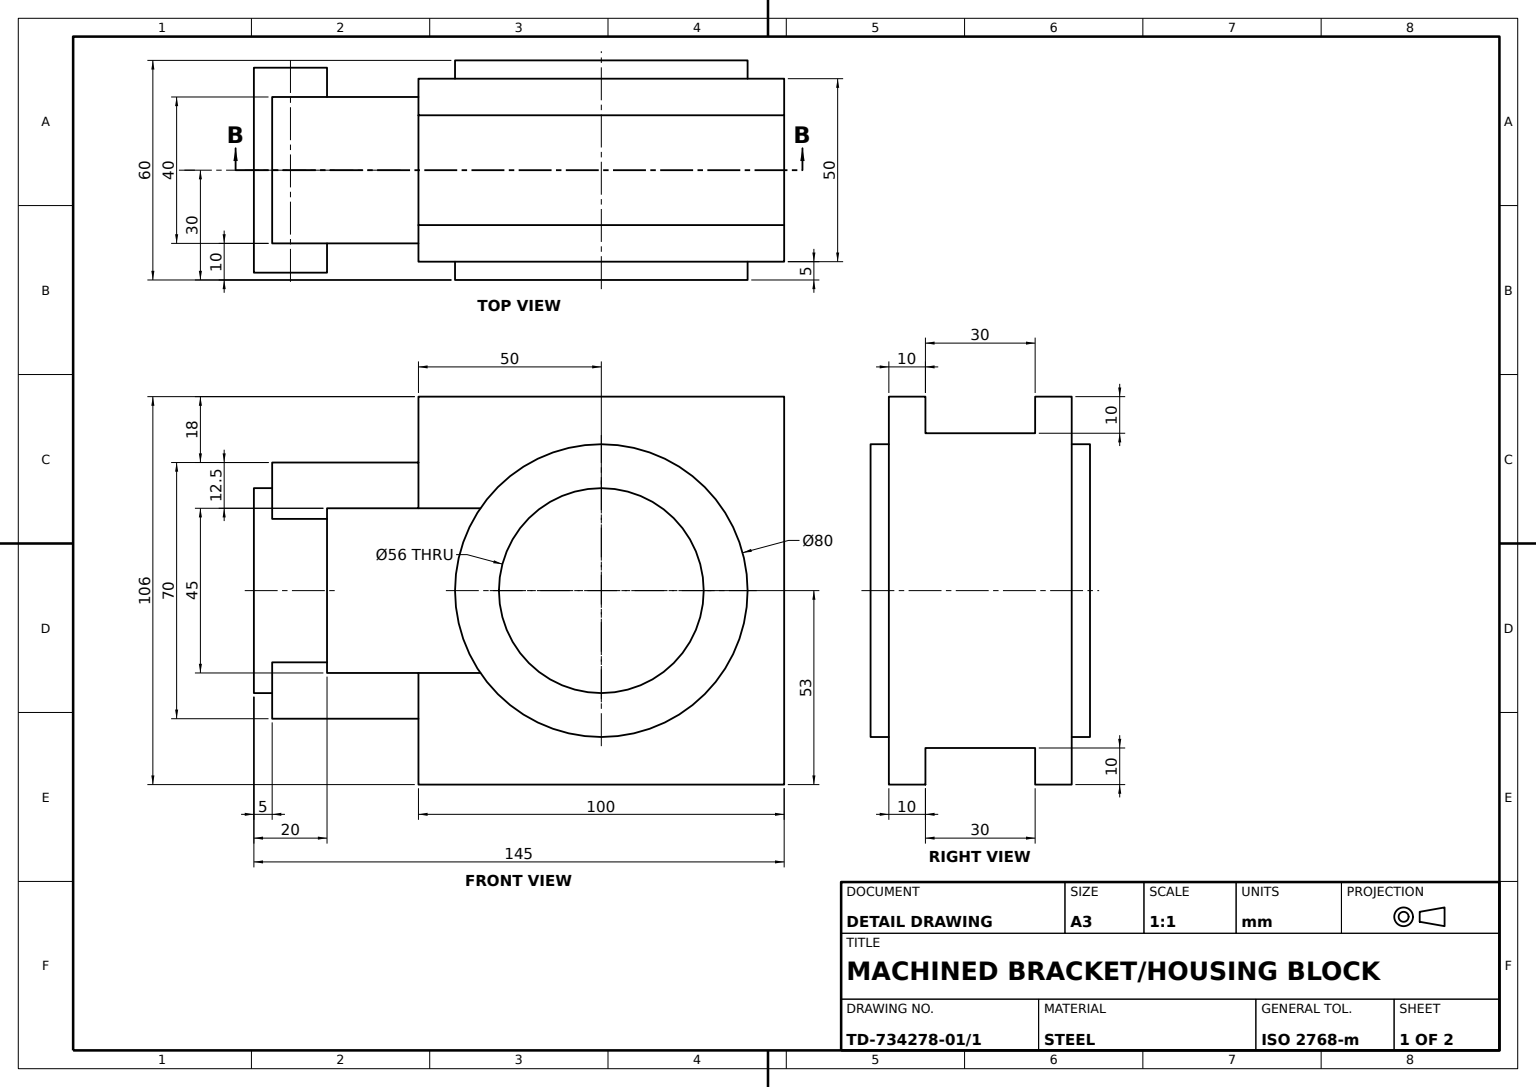
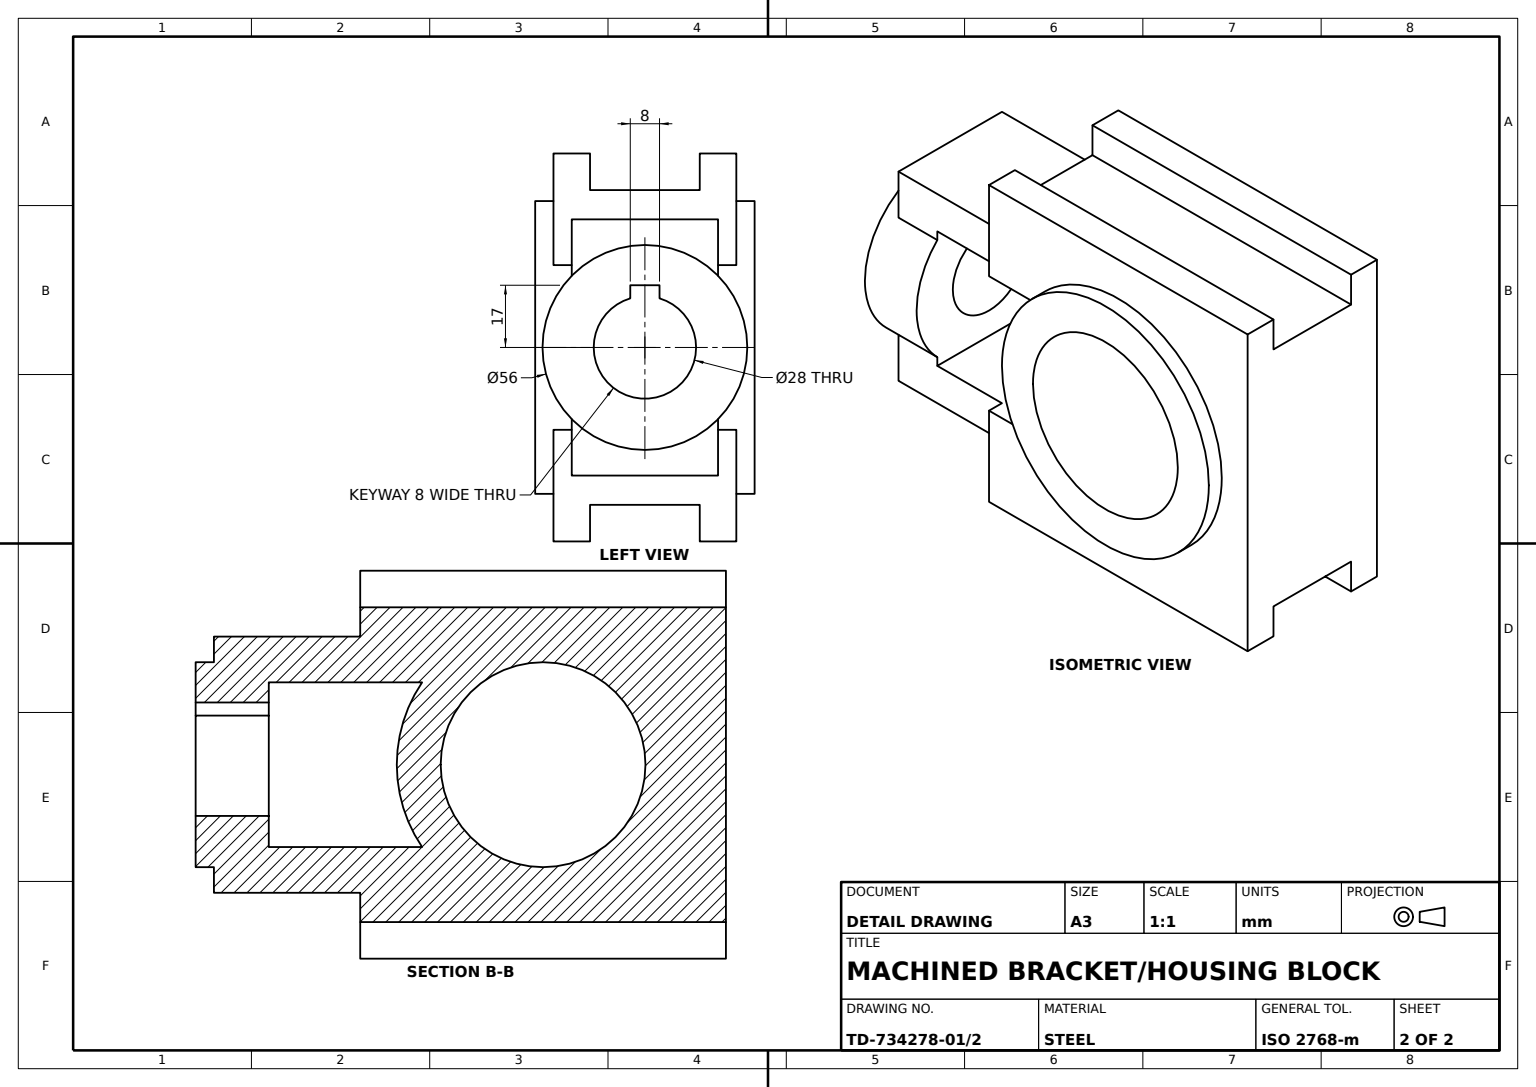
SolidWorks part; units mm, degrees
material "Plain Carbon Steel"
ref_plane "Front Plane" through (0, 0, 0) normal (0, 0, 1) x (1, 0, 0)
ref_plane "Top Plane" through (0, 0, 0) normal (0, 1, 0) x (1, 0, 0)
ref_plane "Right Plane" through (0, 0, 0) normal (1, 0, 0) x (0, 0, -1)
sketch "Base Block Profile" plane through (0, 0, 0) normal (1, 0, 0) x (0, 0, -1)
  line L1 (50, 0) -> (50, 53)
  line L2 (50, 53) -> (-50, 53)
  line L3 (-50, 53) -> (-50, -53)
  line L4 (-50, -53) -> (50, -53)
  line L5 (50, -53) -> (50, 0)
  dimension "D1" = 100
  dimension "D2" = 106
  dimension "D3" = 50
extrude "Base Block" add sketch "Base Block Profile" against normal blind 50
sketch "Body Recess Profile" plane through (0, 0, 0) normal (1, 0, 0) x (0, 0, -1)
  line L0 (-50, 0) -> (-50, 22.5)
  line L1 (50, -53) -> (50, 53) construction
  line L2 (-50, 53) -> (-50, -53) construction
  line L3 (-50, 0) -> (-50, -22.5)
  line L4 (-50, 22.5) -> (-33.0719, 22.5)
  line L5 (-50, -22.5) -> (-33.0719, -22.5)
  arc A0 (-33.0719, -22.5) -> (-33.0719, 22.5) centre (0, 0) ccw
  dimension "D1" = 40
  dimension "D2" = 83.0719
extrude "Body Recess Cut" cut sketch "Body Recess Profile" against normal blind 50
sketch "Bearing Hub Profile" plane through (0, 0, 0) normal (1, 0, 0) x (0, 0, -1)
  circle A0 centre (0, 0) radius 40
  dimension "D1" = 80
extrude "Bearing Hub Boss" add sketch "Bearing Hub Profile" against normal blind 50
sketch "Hub Flange Profile" plane through (0, 0, 0) normal (1, 0, 0) x (0, 0, -1)
  circle A0 centre (0, 0) radius 40
  dimension "D1" = 80
extrude "Hub Flange Boss" add sketch "Hub Flange Profile" along normal blind 5
sketch "Main Bore Profile" plane through (5, 0, 0) normal (1, 0, 0) x (0, 0, -1)
  circle A0 centre (0, 0) radius 28
  dimension "D1" = 56
extrude "Main Bore Cut" cut sketch "Main Bore Profile" against normal blind 113
sketch "Top Slot Profile" plane through (0, 53, 0) normal (0, 1, 0) x (1, 0, 0)
  line L0 (0, 50) -> (0, -50) construction
  line L1 (-50, 50) -> (0, 50) construction
  line L2 (-40, 50) -> (-40, -50)
  line L3 (-50, -50) -> (0, -50) construction
  line L4 (-40, -50) -> (-10, -50)
  line L5 (-10, -50) -> (-10, 50)
  line L6 (-10, 50) -> (-40, 50)
  dimension "D1" = 10
  dimension "D2" = 40
extrude "Top Slot Cut" cut sketch "Top Slot Profile" against normal blind 10
ref_plane "Plane2" through (-5, 0, 0) normal (1, 0, 0) x (0, 0, -1)
sketch "Side Arm Profile" plane through (-5, 0, 0) normal (1, 0, 0) x (0, 0, -1)
  line L0 (-90, 0) -> (-90, 35)
  line L1 (-50, 22.5) -> (-75, 22.5)
  line L2 (-75, 22.5) -> (-75, -22.5)
  line L3 (-90, 35) -> (-50, 35)
  line L4 (-50, 53) -> (-50, 22.5) construction
  line L5 (-90, 0) -> (-90, -35)
  line L6 (-90, -35) -> (-50, -35)
  line L7 (-50, -22.5) -> (-50, -53) construction
  line L8 (-50, -35) -> (-50, -22.5)
  line L9 (-75, -22.5) -> (-50, -22.5)
  line L17 (-33.0719, -22.5) -> (-50, -22.5)
  line L18 (-50, -22.5) -> (-50, -53)
  line L19 (-50, -53) -> (50, -53)
  line L20 (50, -53) -> (50, 53)
  line L21 (50, 53) -> (-50, 53)
  line L22 (-50, 53) -> (-50, 22.5)
  line L23 (-50, 22.5) -> (-33.0719, 22.5)
  line L29 (-50, 35) -> (-50, 22.5)
  arc A2 (-33.0719, -22.5) -> (-33.0719, 22.5) centre (0, 0) ccw
  dimension "D1" = 0
  dimension "D2" = 15
  dimension "D3" = 40
  dimension "D4" = 12.5
extrude "Side Arm Boss" add sketch "Side Arm Profile" against normal blind 40
sketch "Arm Hole Profile" plane through (0, 0, 90) normal (0, 0, 1) x (1, 0, 0)
  line L0 (-5, 35) -> (-5, -35) construction
  line L1 (-45, 35) -> (-5, 35) construction
  circle A0 centre (-25, 0) radius 28
  dimension "D1" = 56
  dimension "D2" = 20
  dimension "D3" = 35
extrude "Arm Hole Cut" cut sketch "Arm Hole Profile" against normal blind 15
sketch "Shaft Hub Profile" plane through (0, 0, 90) normal (0, 0, 1) x (1, 0, 0)
  circle A0 centre (-25, 0) radius 28
  dimension "D1" = 56
extrude "Shaft Hub Boss" add sketch "Shaft Hub Profile" along normal blind 5 and the other way blind 15
sketch "Keyed Bore Profile" plane through (0, 0, 95) normal (0, 0, 1) x (1, 0, 0)
  line L1 (-21, 13.4164) -> (-21, 17)
  line L2 (-21, 17) -> (-29, 17)
  line L3 (-29, 17) -> (-29, 13.4164)
  arc A0 (-29, 13.4164) -> (-21, 13.4164) centre (-25, 0) ccw
  circle A1 centre (-25, 0) radius 28 construction
  dimension "D1" = 14
  dimension "D2" = 4
  dimension "D3" = 17
extrude "Keyed Bore Cut" cut sketch "Keyed Bore Profile" against normal blind 30
sketch "Rear Ring Profile" plane through (-50, 0, 0) normal (-1, 0, 0) x (0, 0, 1)
  circle A0 centre (0, 0) radius 40
  dimension "D1" = 80
extrude "Rear Ring Boss" add sketch "Rear Ring Profile" along normal blind 5
sketch "Through Bore Profile" plane through (5, 0, 0) normal (1, 0, 0) x (0, 0, -1)
  circle A0 centre (0, 0) radius 28
  dimension "D1" = 56
extrude "Through Bore Cut" cut sketch "Through Bore Profile" against normal blind 194
sketch "Second Slot Profile" plane through (0, -53, 0) normal (0, -1, 0) x (1, 0, 0)
  line L1 (-50, 50) -> (0, 50) construction
  line L2 (-40, 50) -> (-40, -50)
  line L3 (-40, -50) -> (-10, -50)
  line L4 (-50, -50) -> (0, -50) construction
  line L5 (-10, -50) -> (-10, 50)
  line L6 (-10, 50) -> (-40, 50)
  dimension "D1" = 10
extrude "Second Slot Cut" cut sketch "Second Slot Profile" against normal blind 10
